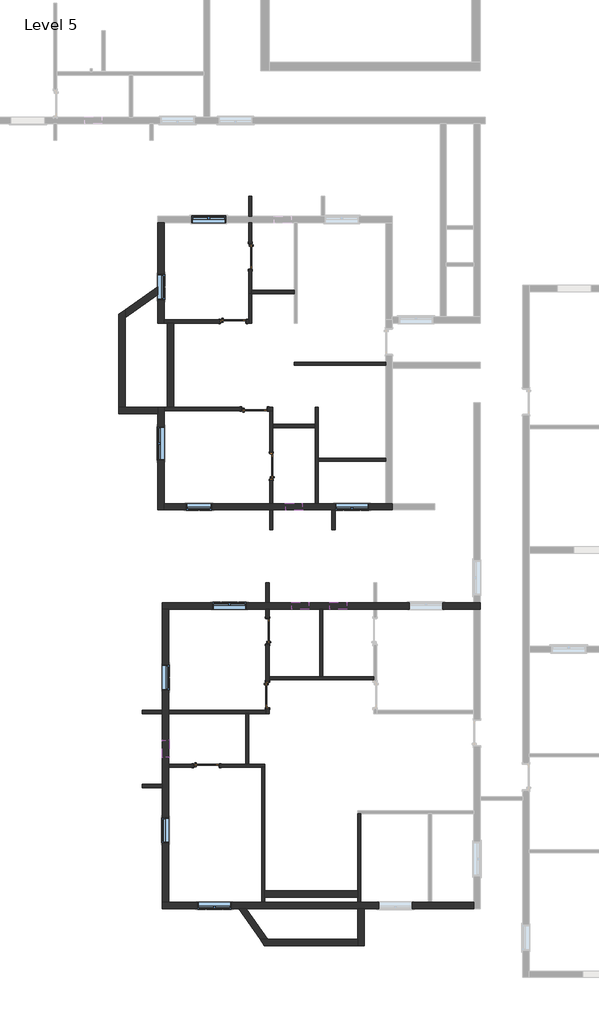
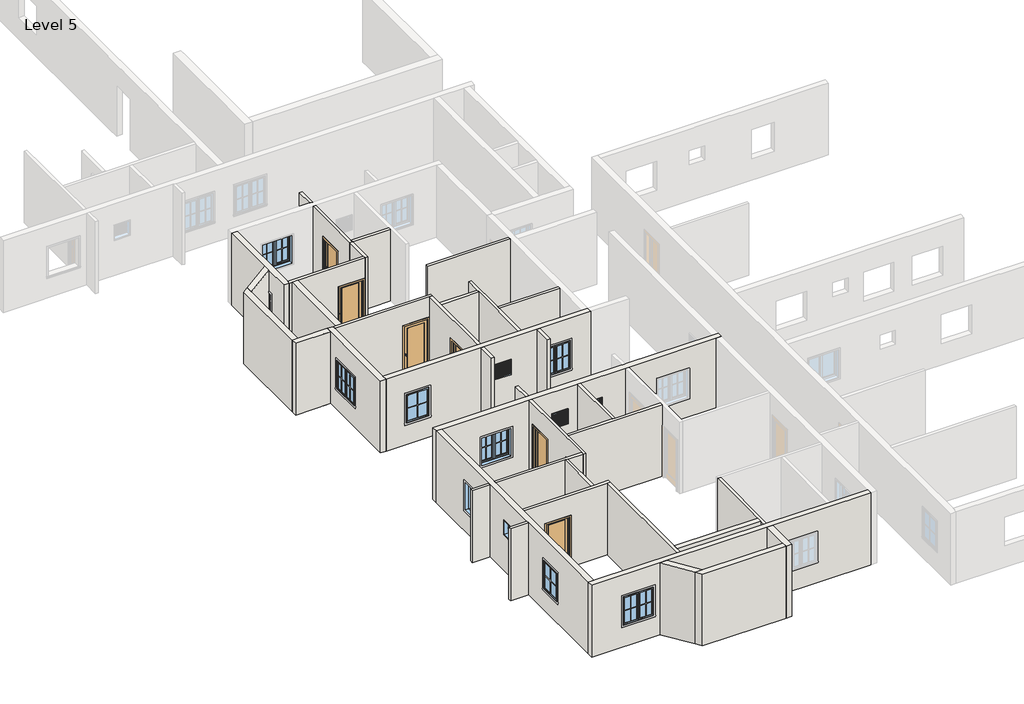
# One storey, part 1 of 7: 39 walls, 13 windows, 7 doors.
# Revit data of these elements (continued)
# Element 50 (IfcWindow, "Window-Awning-Single : 36\" x 48\"") (continued)
#   Interior Wall Closure = 0' - 2 1/4"
#   Frame Extension = 0' - 0 1/4"
#   Exterior Wall Closure = 0' - 1 1/4"
#   Interior Trim Visibility = yes
#   Exterior Trim Visibility = yes
#   Phase Created = New Construction
#   Materials on its faces: "Wood - Stained", "Glass", "Clad - White"
# Element 51 (IfcWindow, "Window-Casement-Double : 4' x 4'")
#   Mark = "118"
#   Window Inset = 0' - 0"
#   Interior Wall Closure = 0' - 2 1/4"
#   Frame Extension = 0' - 0 1/4"
#   Exterior Wall Closure = 0' - 1 1/4"
#   Interior Trim Visibility = yes
#   Exterior Trim Visibility = yes
#   Phase Created = New Construction
#   Materials on its faces: "Wood - Stained", "Glass", "Clad - White"
# Element 52 (IfcWindow, "Window-Casement-Double : 4' x 4'")
#   Mark = "120"
#   Window Inset = 0' - 0"
#   Interior Wall Closure = 0' - 2 1/4"
#   Frame Extension = 0' - 0 1/4"
#   Exterior Wall Closure = 0' - 1 1/4"
#   Interior Trim Visibility = yes
#   Exterior Trim Visibility = yes
#   Phase Created = New Construction
#   Materials on its faces: "Wood - Stained", "Glass", "Clad - White"
# Element 53 (IfcWindow, "Window-Casement-Double : 4' x 4'")
#   Mark = "122"
#   Window Inset = 0' - 0"
#   Interior Wall Closure = 0' - 2 1/4"
#   Frame Extension = 0' - 0 1/4"
#   Exterior Wall Closure = 0' - 1 1/4"
#   Interior Trim Visibility = yes
#   Exterior Trim Visibility = yes
#   Phase Created = New Construction
#   Materials on its faces: "Wood - Stained", "Glass", "Clad - White"
# Element 54 (IfcWindow, "Window-Casement-Double : 4' x 4'")
#   Mark = "123"
#   Window Inset = 0' - 0"
#   Interior Wall Closure = 0' - 2 1/4"
#   Frame Extension = 0' - 0 1/4"
#   Exterior Wall Closure = 0' - 1 1/4"
#   Interior Trim Visibility = yes
#   Exterior Trim Visibility = yes
#   Phase Created = New Construction
#   Materials on its faces: "Wood - Stained", "Glass", "Clad - White"
# Element 55 (IfcWindow, "Window-Casement-Double : 4' x 4'")
#   Mark = "125"
#   Window Inset = 0' - 0"
#   Interior Wall Closure = 0' - 2 1/4"
#   Frame Extension = 0' - 0 1/4"
#   Exterior Wall Closure = 0' - 1 1/4"
#   Interior Trim Visibility = yes
#   Exterior Trim Visibility = yes
#   Phase Created = New Construction
#   Materials on its faces: "Wood - Stained", "Glass", "Clad - White"
# Element 56 (IfcWindow, "Window-Louvers : 24\" x 24\"")
#   Mark = "74"
#   Blade Width = 1' - 10 1/2"
#   Phase Created = New Construction
#   Materials on its faces: "Birch"
# Element 57 (IfcWindow, "Window-Louvers : 24\" x 24\"")
#   Mark = "77"
#   Blade Width = 1' - 10 1/2"
#   Phase Created = New Construction
#   Materials on its faces: "Birch"
# Element 58 (IfcWindow, "Window-Louvers : 24\" x 24\"")
#   Mark = "78"
#   Blade Width = 1' - 10 1/2"
#   Phase Created = New Construction
#   Materials on its faces: "Birch"
# Element 59 (IfcWindow, "Window-Louvers : 24\" x 24\"")
#   Mark = "80"
#   Blade Width = 1' - 10 1/2"
#   Phase Created = New Construction
#   Materials on its faces: "Birch"
# Materials
#   "Cherry": class "Wood", colour RGB 226 177 128, transparency 0, Description = "Prunus Serotina", Cost = 0
#   "Aluminum": class "Metal", colour RGB 247 247 247, transparency 0, Description = "Aluminum 6061", Cost = 0
#   "Wood - Stained": class "Wood", colour RGB 224 178 126, transparency 0, Cost = 0
#   "Glass": class "Glass", colour RGB 0 128 192, transparency 0.75, Description = "Soda Lime Glass", Cost = 0
#   "Clad - White": class "Wood", colour RGB 242 242 238, transparency 0, Cost = 0
#   "Birch": class "Wood", colour RGB 224 178 126, transparency 0, Description = "Betula Alleghaniensis", Cost = 0
#   "Default Wall": colour RGB 128 128 128, transparency 0, Cost = 0
